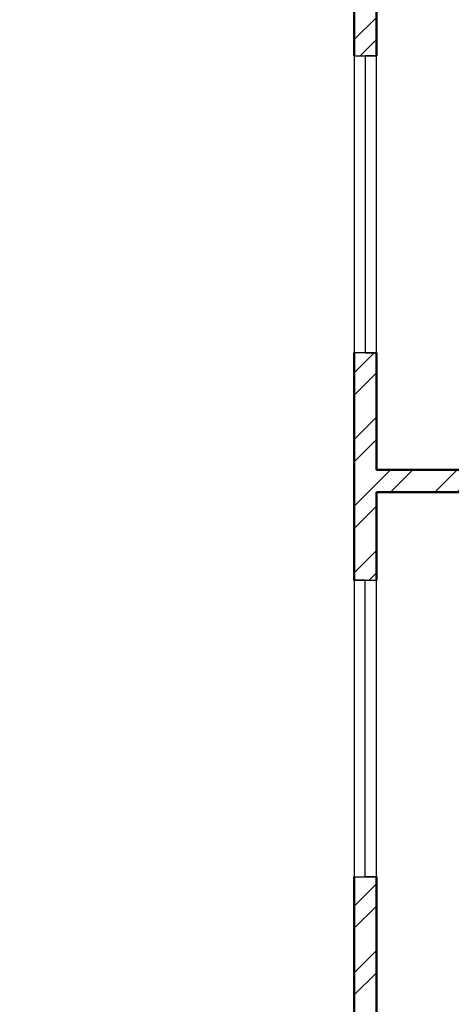
# Model space of a CAD drawing. Units: inches. Extents: x 963 to 2075, y 289 to 2657.
# Tile 13 of 98: x 1091 to 1179, y 1718 to 1917. Entities that reach past the tile are written whole.
import ezdxf

# ---------------------------------------------------------------- set-up
doc = ezdxf.new("R2010")
doc.units = ezdxf.units.IN
for name, color, linetype, lineweight in [('A-GLAZ', 3, 'Continuous', 25), ('A-WALL', 7, 'Continuous', 50), ('A-WALL-PATT', 8, 'Continuous', 13)]:
    doc.layers.add(name, color=color, linetype=linetype, lineweight=lineweight)

msp = doc.modelspace()

# ---------------------------------------------------------------- hatches: boundary and pattern name
at = {"layer": 'A-WALL-PATT'}
h = msp.add_hatch(dxfattribs=at)
h.set_pattern_fill('ANSI32', color=256)
h.paths.add_polyline_path([(1473.61, 2163.07), (1473.61, 2165.32), (1376.42, 2165.32), (1376.42, 2227.98), (1371.92, 2227.98), (1371.92, 2214.82), (1368.41, 2214.82), (1368.41, 2210.32), (1371.92, 2210.32), (1371.92, 2160.82), (1395.92, 2160.82), (1395.92, 2090.32), (1217.34, 2090.32), (1217.34, 2085.82), (1395.92, 2085.82), (1458.92, 2085.82), (1458.92, 2108.32), (1454.42, 2108.32), (1454.42, 2090.32), (1400.42, 2090.32), (1400.42, 2160.82), (1473.61, 2160.82)])
h.paths.add_polyline_path([(1649.42, 2210.32), (1653.23, 2210.32), (1653.23, 2214.82), (1649.42, 2214.82), (1649.42, 2227.98), (1644.92, 2227.98), (1644.92, 2165.32), (1550.1, 2165.32), (1550.1, 2160.82), (1620.92, 2160.82), (1620.92, 2112.82), (1555.45, 2112.82), (1555.45, 2108.32), (1584.33, 2108.32), (1584.33, 2084.92), (1588.83, 2084.92), (1588.83, 2108.32), (1625.42, 2108.32), (1667.95, 2108.32), (1667.95, 2022.67), (1588.83, 2022.67), (1588.83, 2047.41), (1584.33, 2047.41), (1584.33, 1996), (1588.83, 1996), (1588.83, 2018.32), (1667.95, 2018.17), (1667.95, 1928.32), (1625.42, 1928.32), (1625.42, 1923.82), (1672.45, 1923.82), (1672.45, 1928.32), (1672.45, 1946.66), (1785.45, 1946.66), (1785.45, 1951.16), (1743.03, 1951.16), (1743.03, 2017.92), (1841.42, 2017.92), (1841.42, 2014.77), (1845.92, 2014.77), (1845.92, 2017.92), (1905.92, 2017.92), (1905.92, 1987.51), (1910.42, 1987.51), (1910.42, 2022.42), (1910.42, 2068.52), (1905.92, 2068.52), (1905.92, 2022.42), (1845.92, 2022.42), (1845.92, 2025.85), (1843.67, 2025.85), (1841.42, 2025.85), (1841.42, 2022.42), (1743.03, 2022.42), (1743.03, 2084.03), (1768.45, 2084.03), (1785.45, 2084.03), (1785.45, 2088.53), (1672.45, 2088.53), (1672.45, 2112.82), (1667.95, 2112.82), (1625.42, 2112.82), (1625.42, 2160.82), (1649.42, 2160.82)])
h.paths.add_polyline_path([(1672.45, 2084.03), (1738.53, 2084.03), (1738.53, 1951.16), (1672.45, 1951.16)], flags=16)
h.paths.add_polyline_path([(1672.45, 2084.03), (1738.53, 2084.03), (1705.49, 2017.6)], flags=0)
h.paths.add_polyline_path([(1262.77, 2085.82), (1258.27, 2085.82), (1258.27, 2023.28), (1184.42, 2023.28), (1184.42, 2018.78), (1258.27, 2018.78), (1258.27, 1950.82), (1262.77, 1950.82)])
h.paths.add_polyline_path([(1312.27, 2085.82), (1307.77, 2085.82), (1307.77, 1950.82), (1312.27, 1950.82)])
h.paths.add_polyline_path([(1458.92, 1950.82), (1395.92, 1950.82), (1216.57, 1950.82), (1216.57, 1946.32), (1346.42, 1946.32), (1395.92, 1946.32), (1395.92, 1875.82), (1371.92, 1875.82), (1371.92, 1826.32), (1368.93, 1826.32), (1368.93, 1821.82), (1371.92, 1821.82), (1371.92, 1813.62), (1376.42, 1813.62), (1376.42, 1871.32), (1474.5, 1871.32), (1474.5, 1873.57), (1474.5, 1875.82), (1400.42, 1875.82), (1400.42, 1946.32), (1454.42, 1946.32), (1454.42, 1928.32), (1458.92, 1928.32)])
h.paths.add_polyline_path([(1184.42, 2120.78), (1167.92, 2120.78), (1167.92, 2134.81), (1165.67, 2134.81), (1163.42, 2134.81), (1163.42, 2120.78), (1119.92, 2120.78), (1119.92, 2098.1), (1124.42, 2098.1), (1124.42, 2116.28), (1167.92, 2116.28), (1179.92, 2116.28), (1179.92, 2045.92), (1184.42, 2045.92), (1184.42, 2090.32), (1184.42, 2116.28)])
h.paths.add_polyline_path([(1124.42, 2018.78), (1179.92, 2018.78), (1179.92, 2016.29), (1184.42, 2016.29), (1184.42, 2023.28), (1184.42, 2026.59), (1182.17, 2026.59), (1179.92, 2026.59), (1179.92, 2023.28), (1124.42, 2023.28), (1124.42, 2074.1), (1119.92, 2074.1), (1119.92, 2018.78), (1119.92, 1979.63), (1124.42, 1979.63)])
h.paths.add_polyline_path([(1184.42, 1925.78), (1184.42, 1946.32), (1184.42, 1996.07), (1182.17, 1996.07), (1179.92, 1996.07), (1179.92, 1925.78), (1124.42, 1925.78), (1124.42, 1955.63), (1119.92, 1955.5), (1119.92, 1921.28), (1158.92, 1921.28), (1158.92, 1909.98), (1163.42, 1909.98), (1163.42, 1921.28), (1184.42, 1921.28)])
h.paths.add_polyline_path([(1341.45, 1826.32), (1163.42, 1826.32), (1163.42, 1849.98), (1158.92, 1849.98), (1158.92, 1821.82), (1158.92, 1804.03), (1163.42, 1804.03), (1163.42, 1821.82), (1341.45, 1821.82)])
h.paths.add_polyline_path([(1222.98, 1713.82), (1163.42, 1713.82), (1163.42, 1744.03), (1161.17, 1744.03), (1158.92, 1744.03), (1158.92, 1713.82), (1119.92, 1713.82), (1119.92, 1694.65), (1124.42, 1694.65), (1124.42, 1709.32), (1158.92, 1709.32), (1222.98, 1709.32)])
h.paths.add_polyline_path([(1328.42, 1713.82), (1252.04, 1713.82), (1252.04, 1711.57), (1252.04, 1709.32), (1256.42, 1709.32), (1256.42, 1547.32), (1232.94, 1547.32), (1232.94, 1545.07), (1232.94, 1542.82), (1292.42, 1542.82), (1292.42, 1527.63), (1296.92, 1527.63), (1296.92, 1542.82), (1299.46, 1542.82), (1299.46, 1547.32), (1260.92, 1547.32), (1260.92, 1658.32), (1343.66, 1658.32), (1343.66, 1660.57), (1343.66, 1662.82), (1328.42, 1662.82), (1328.42, 1676.59), (1327.4, 1676.59), (1323.92, 1676.59), (1323.92, 1662.82), (1260.92, 1662.82), (1260.92, 1709.32), (1323.92, 1709.32), (1323.92, 1699.85), (1328.42, 1699.85)])
h.paths.add_polyline_path([(1649.42, 1875.82), (1625.42, 1875.82), (1625.42, 1928.32), (1620.92, 1928.32), (1588.83, 1928.32), (1588.83, 1950.59), (1584.33, 1950.59), (1584.33, 1928.32), (1555.45, 1928.32), (1555.45, 1923.82), (1620.92, 1923.82), (1620.92, 1875.82), (1548.95, 1875.82), (1548.95, 1873.57), (1548.95, 1871.32), (1644.92, 1871.32), (1644.92, 1813.62), (1649.42, 1813.62), (1649.42, 1821.82), (1652.04, 1821.82), (1652.04, 1824.07), (1652.04, 1826.32), (1649.42, 1826.32)])
h.paths.add_polyline_path([(1512.92, 1871.32), (1516.48, 1871.32), (1516.48, 1875.82), (1512.92, 1875.82), (1512.92, 1923.82), (1512.92, 1928.32), (1512.92, 1930.83), (1508.42, 1930.83), (1508.42, 1875.82), (1504.41, 1875.82), (1504.41, 1871.32), (1508.42, 1871.32), (1508.42, 1713.82), (1376.42, 1713.82), (1376.42, 1743.32), (1371.92, 1743.32), (1371.92, 1709.32), (1371.92, 1706.01), (1376.42, 1706.01), (1376.42, 1709.32), (1508.42, 1709.32), (1508.42, 1547.32), (1501.87, 1547.32), (1501.87, 1542.82), (1508.42, 1542.82), (1508.42, 1482.82), (1508.42, 1436.32), (1512.92, 1436.32), (1512.92, 1542.82), (1519.32, 1542.82), (1519.32, 1545.07), (1519.32, 1547.32), (1512.92, 1547.32), (1512.92, 1709.32), (1644.92, 1709.32), (1644.92, 1707.55), (1649.42, 1707.55), (1649.42, 1709.32), (1649.42, 1743.32), (1644.92, 1743.32), (1644.92, 1713.82), (1512.92, 1713.82)])
h.paths.add_polyline_path([(1129.88, 1545.07), (1129.88, 1547.32), (1124.42, 1547.32), (1095.92, 1547.32), (1095.92, 1614.82), (1124.42, 1614.82), (1124.42, 1619.32), (1095.92, 1619.32), (1091.42, 1619.32), (1091.42, 1542.82), (1095.92, 1542.82), (1119.92, 1542.82), (1129.88, 1542.82)])
h.paths.add_polyline_path([(1208.42, 1542.82), (1211.74, 1542.82), (1211.74, 1547.32), (1198.85, 1547.32), (1198.85, 1542.82), (1203.92, 1542.82), (1203.92, 1478.32), (1208.42, 1478.32), (1296.92, 1478.32), (1296.92, 1503.63), (1292.42, 1503.63), (1292.42, 1482.82), (1208.42, 1482.82)])
h.paths.add_polyline_path([(1430.42, 1542.82), (1435.7, 1542.82), (1435.7, 1545.07), (1435.7, 1547.32), (1422.66, 1547.32), (1422.66, 1545.07), (1422.66, 1542.82), (1425.92, 1542.82), (1425.92, 1482.86), (1341.92, 1482.86), (1341.92, 1502.73), (1337.42, 1502.73), (1337.42, 1478.36), (1425.92, 1478.36), (1425.92, 1440.82), (1425.92, 1436.32), (1430.42, 1436.32)])
h.paths.add_polyline_path([(1698.48, 2004.26), (1727.69, 2004.26), (1727.69, 2022.92), (1698.48, 2022.92)], flags=8)

# ---------------------------------------------------------------- linework, layer by layer
at = {"layer": 'A-GLAZ'}
for p, q in [((1158.92, 1909.98), (1163.42, 1909.98)), ((1158.92, 1909.98), (1158.92, 1849.98)), ((1163.42, 1909.98), (1161.17, 1909.98)), ((1161.17, 1909.98), (1161.17, 1849.98)), ((1163.42, 1849.98), (1163.42, 1909.98)), ((1163.42, 1849.98), (1158.92, 1849.98)), ((1161.17, 1849.98), (1163.42, 1849.98)), ((1161.17, 1804.03), (1158.92, 1804.03)), ((1158.92, 1804.03), (1163.42, 1804.03)), ((1158.92, 1804.03), (1158.92, 1744.03)), ((1161.17, 1744.03), (1161.17, 1804.03)), ((1163.42, 1744.03), (1163.42, 1804.03)), ((1158.92, 1744.03), (1163.42, 1744.03)), ((1163.42, 1744.03), (1161.17, 1744.03))]:
    msp.add_line(p, q, dxfattribs=at)
at = {"layer": 'A-WALL'}
for p, q in [((1158.92, 1909.98), (1158.92, 1921.28)), ((1163.42, 1921.28), (1163.42, 1909.98)), ((1158.92, 1821.82), (1158.92, 1849.98)), ((1163.42, 1849.98), (1163.42, 1826.32)), ((1163.42, 1826.32), (1342.58, 1826.32)), ((1158.92, 1804.03), (1158.92, 1821.82)), ((1163.42, 1821.82), (1163.42, 1804.03)), ((1341.45, 1821.82), (1163.42, 1821.82)), ((1158.92, 1713.82), (1158.92, 1744.03)), ((1163.42, 1744.03), (1163.42, 1713.82))]:
    msp.add_line(p, q, dxfattribs=at)

doc.saveas('drawing.dxf')
